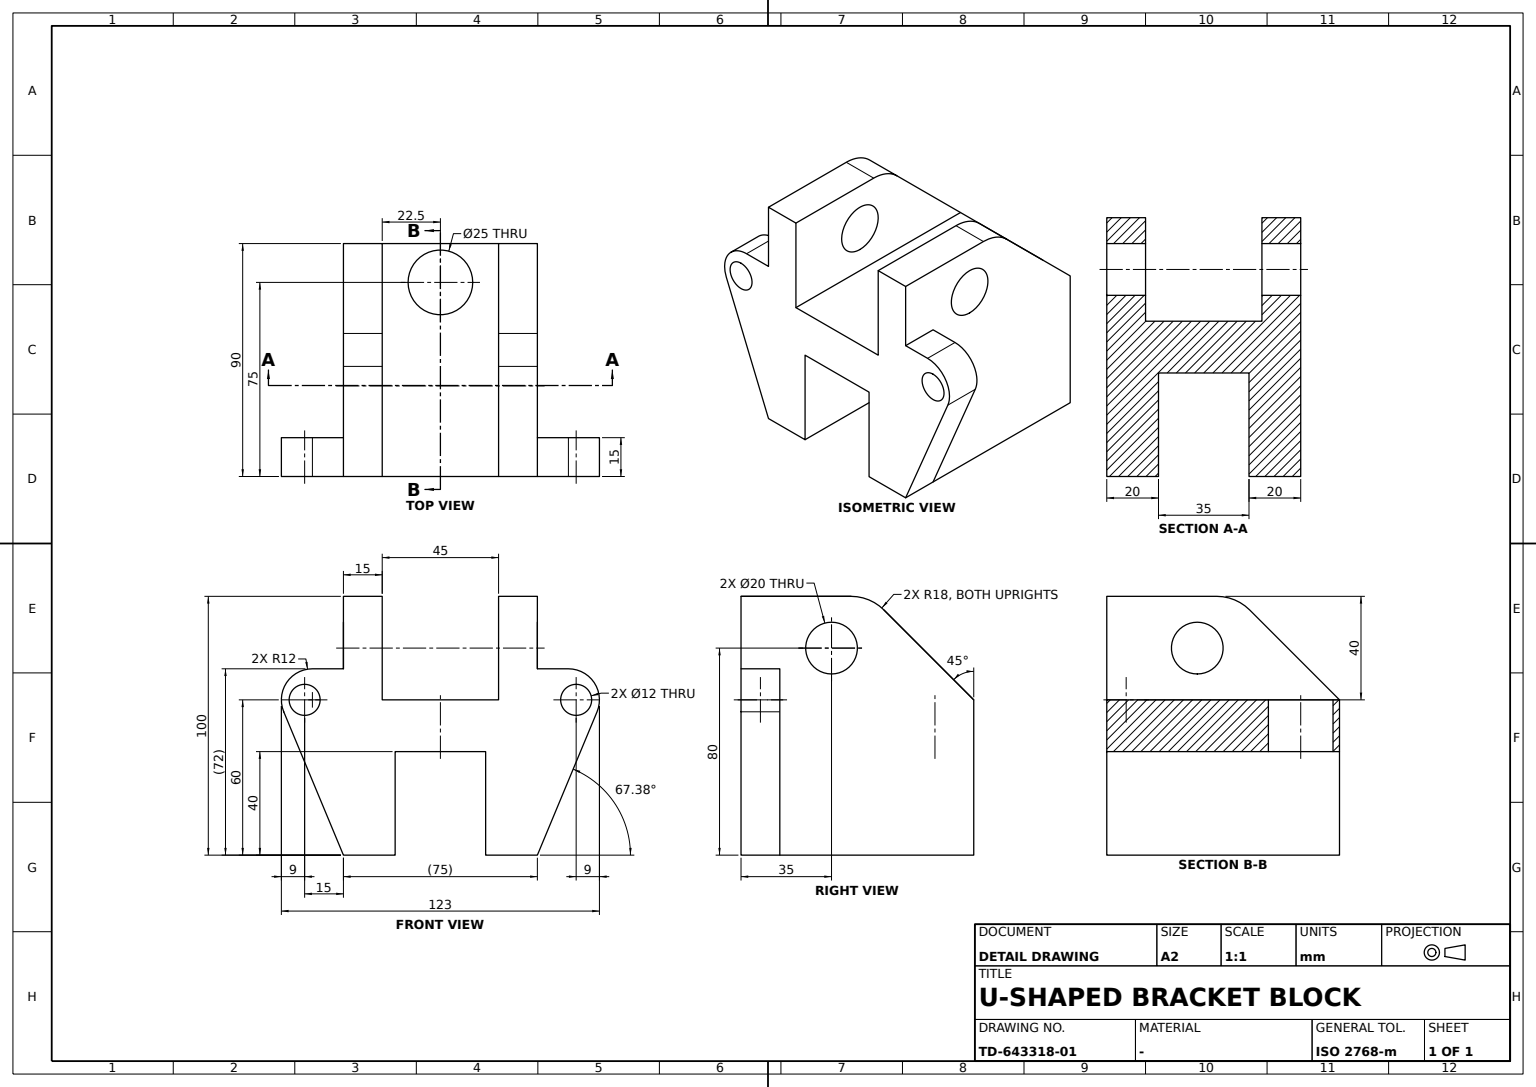
CATIA V5 part; units mm, degrees
sketch "Sketch1" plane through (0, 0, 0) normal (0, 1, 0) x (-1, 0, 0)
  line L0 (0, 0) -> (-17.5, 0)
  line L1 (-17.5, 0) -> (-17.5, -40)
  line L2 (-17.5, -40) -> (-37.5, -40)
  line L3 (-37.5, -40) -> (-37.5, 20)
  line L4 (-37.5, 20) -> (37.5, 20)
  line L5 (37.5, 20) -> (37.5, -40)
  line L6 (37.5, -40) -> (17.5, -40)
  line L7 (17.5, -40) -> (17.5, 0)
  point P0 (17.5, 0)
  line L8 (17.5, 0) -> (0, 0)
  dimension "length L3" = 60
  dimension "length L5" = 60
  dimension "distance L1 L7" = 35
  dimension "distance L3 L5" = 75
  dimension "length L1" = 40
  constraint horizontal L0 x-axis
  constraint horizontal L2 x-axis
  constraint horizontal L4 x-axis
  constraint horizontal L6 x-axis
  constraint horizontal L8 x-axis
  constraint vertical L1 y-axis
  constraint vertical L3 y-axis
  constraint vertical L5 y-axis
  constraint vertical L7 y-axis
  constraint coincidence P0 x-axis
  constraint symmetry L3 L5 y-axis
  constraint symmetry L1 L7 y-axis
extrude "Pad1" add sketch "Sketch1" along normal mid plane 90
sketch "Sketch2" plane through (37.5, 0, 0) normal (1, 0, 0) x (0, 1, 0)
  line L0 (-45, 20) -> (-45, 60)
  line L1 (-45, 60) -> (5, 60)
  line L2 (5, 60) -> (45, 20)
  point P0 (45, 20)
  line L3 (45, 20) -> (-45, 20)
  line L4 (-45, 20) -> (45, 20) construction
  line L5 (-45, 20) -> (-45, -40) construction
  circle A0 centre (-10, 40) radius 10
  point P1 (-10, 40)
  line L6 (45, 20) -> (45, -40) construction
  dimension "length L0" = 40
  dimension "length L1" = 50
  dimension "radius A0" = 10
  dimension "distance L0 P1" = 35
  dimension "distance L3 P1" = 20
  constraint vertical L0 y-axis
  constraint horizontal L1 x-axis
  constraint horizontal L3 x-axis
  constraint coincidence L3 L4
  constraint coincidence L0 L5
  constraint coincidence P0 L6
extrude "Pad2" add sketch "Sketch2" against normal blind 15
mirror "Mirror1" about plane through (0, 0, 0) normal (1, 0, 0) of "Pad2"
fillet "Fillet1" radius 18 2 edges at (30, 5, 60) (-30, 5, 60)
sketch "Sketch3" plane through (0, 0, 20) normal (0, 0, 1) x (0, 1, 0)
  circle A0 centre (30, 0) radius 12.5
  point P0 (30, 0)
  dimension "radius A0" = 12.5
  dimension "distance y axis P0" = 30
  constraint coincidence P0 x-axis
extrude "Pocket1" cut sketch "Sketch3" against normal blind 20
sketch "Sketch4" plane through (0, -45, 0) normal (0, -1, 0) x (1, 0, 0)
  point P0 (37.5, -40)
  line L0 (37.5, -40) -> (37.5, 32)
  line L1 (37.5, 32) -> (67.5, 32)
  line L2 (67.5, 32) -> (37.5, -40)
  circle A0 centre (52.5, 20) radius 6
  point P1 (52.5, 20)
  line L3 (37.5, 20) -> (37.5, -40) construction
  point P2 (37.5, -40)
  line L4 (37.5, -40) -> (17.5, -40) construction
  dimension "length L1" = 30
  dimension "distance L0 P1" = 15
  dimension "length L0" = 72
  dimension "distance L4 P1" = 60
  dimension "radius A0" = 6
  constraint vertical L0 y-axis
  constraint horizontal L1 x-axis
  constraint coincidence L0 L3
  constraint coincidence P0 P2
extrude "Pad3" add sketch "Sketch4" against normal blind 15
fillet "Fillet2" radius 12 1 edges at (67.5, -37.5, 32)
mirror "Mirror2" about plane through (0, 0, 0) normal (1, 0, 0) of "Pad3"
fillet "Fillet3" radius 12 1 edges at (-67.5, -37.5, 32)
